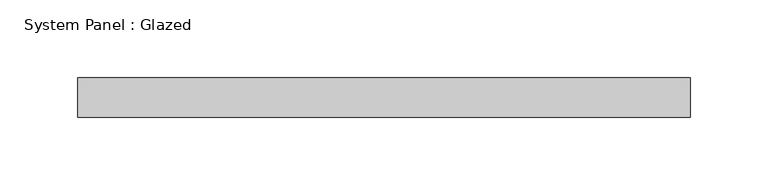
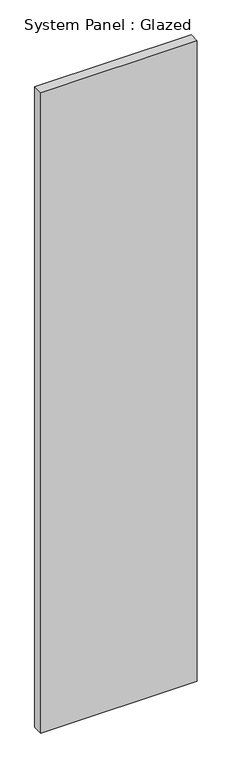
"""IFC4 building model written with IfcOpenShell, lengths in millimetres: plate geometry, System Panel : Glazed."""

from ifc_helpers import new_model, si_unit, origin, origin_with_axes, place, context, project, spatial, polyline, outline, extrude, source, transform, mapped, element, save


def system_panel_glazed_c91192bf(model_context):
    return source(origin(), model_context, "Body", "SweptSolid", [
        extrude(outline(polyline([(196.85, 19.05), (-196.85, 19.05), (-196.85, 44.45), (196.85, 44.45), (196.85, 19.05)])), origin_with_axes(), (0.0, 0.0, 1.0), 1701.8),
    ])


if __name__ == "__main__":
    model = new_model("IFC4")
    model_context = context("Model", 3, world=origin())
    ifc_project = project(units=[si_unit("LENGTHUNIT", "METRE", prefix="MILLI")], contexts=[model_context])
    site = spatial("IfcSite", under=ifc_project)
    building = spatial("IfcBuilding", under=site)
    placement = place(None, origin())
    system_panel_glazed_shape = system_panel_glazed_c91192bf(model_context)
    element("IfcPlate", 1, ObjectType="System Panel : Glazed", at=placement, inside=building, context=model_context, shape_type="MappedRepresentation", body=[
        mapped(system_panel_glazed_shape, transform((0.0, 0.0, 0.0), x_axis=(1.0, 0.0, 0.0), y_axis=(0.0, 1.0, 0.0), z_axis=(0.0, 0.0, 1.0))),
    ])
    save(model, "model.ifc")

# Revit data of these elements
# Type "System Panel : Glazed"
#   Construction Type Id = "GSP4R"
#   Analytic Construction = "1/8 in Pilkington single glazing"
#   Visual Light Transmittance = 0.9
#   Solar Heat Gain Coefficient = 0.86
#   Heat Transfer Coefficient (U) = 1.18115 BTU/(h·ft²·°F)
#   Define Thermal Properties by = 1
# Element 1 (IfcPlate, "System Panel : Glazed")
#   Materials on its faces: "Glass"
# Materials
#   "Glass": class "Glass", colour RGB 0 128 192, transparency 0.75, Description = "Soda Lime Glass", Cost = 0
